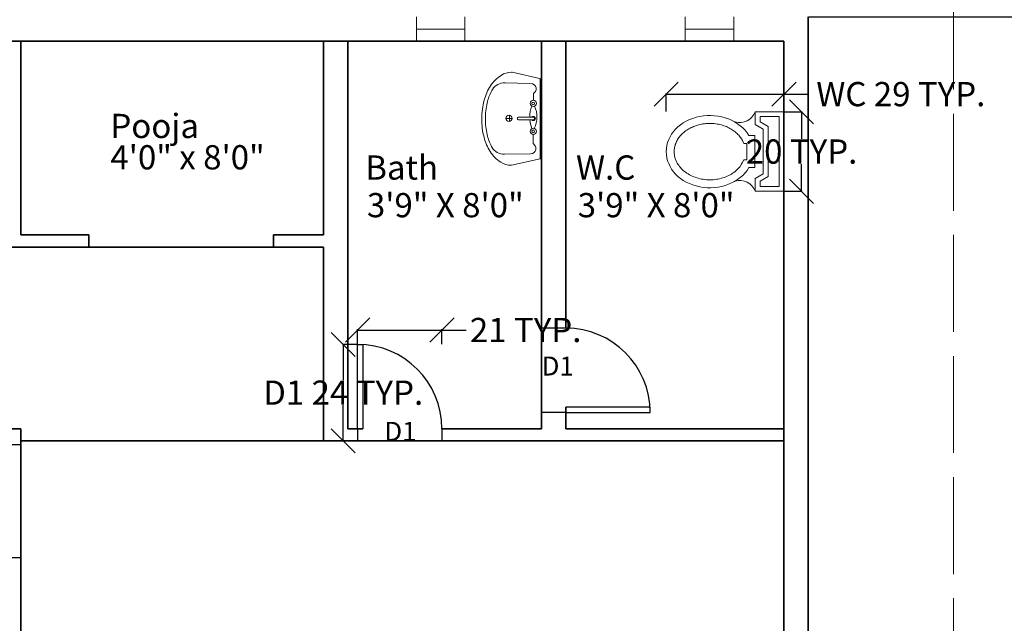
# Model space of a CAD drawing. Units: inches. Extents: x -1198 to -69, y -512 to 437.
# Tile 48 of 50: x -566 to -322, y 113 to 263. Entities that reach past the tile are written whole.
import ezdxf

# ---------------------------------------------------------------- set-up
doc = ezdxf.new("R2010")
doc.units = ezdxf.units.IN
doc.header["$MEASUREMENT"] = 0
doc.linetypes.add('ACAD_ISO02W100', pattern=[15, 12, -3])
for name, color, linetype, lineweight in [('A-ANNO-DIMS', 2, 'Continuous', 18), ('A-ANNO-SYMB', 7, 'Continuous', 18), ('A-AREA-IDEN', 7, 'Continuous', 18), ('A-FLOR-FIXT', 60, 'Continuous', 18), ('A-WALL', 7, 'Continuous', 35), ('C-PROP', 141, 'ACAD_ISO02W100', 18), ('Doors', 140, 'Continuous', 25), ('windows', 160, 'Continuous', 18)]:
    doc.layers.add(name, color=color, linetype=linetype, lineweight=lineweight)
doc.styles.get("Standard").update_dxf_attribs({"font": 'arial.ttf'})
doc.dimstyles.get("Standard").update_dxf_attribs({"dimtxt": 6, "dimasz": 6, "dimexe": 0.18, "dimexo": 0.0625, "dimgap": 0.09, "dimtad": 0, "dimtih": 1, "dimtoh": 1, "dimdec": 0, "dimzin": 0, "dimdsep": 46, "dimlunit": 4, "dimtxsty": 'Standard', "dimblk": 'OBLIQUE', "dimcen": 0.09, "dimadec": 0, "dimazin": 0, "dimtfac": 1, "dimtdec": 0, "dimtofl": 0, "dimtmove": 0, "dimatfit": 3, "dimfxl": 1, "dimtolj": 1, "dimtzin": 0, "dimarcsym": 0})

# ---------------------------------------------------------------- blocks, each defined once
blk = doc.blocks.new('*U4')
for p, q in [((0, 0), (0, -6)), ((28, 0), (28, -6))]:
    blk.add_line(p, q)
blk.add_lwpolyline([(0, 0), (0, 28), (1.75, 28), (1.75, 0)], close=True)
blk.add_arc((0, 0), 28, 0, 90)
blk = doc.blocks.new('A$C7C8779AE')
for p, q in [((0, 0.7405), (0, 0.5605)), ((0.5, 0.7405), (0, 0.7405)), ((0.47, 0.7105), (0.03, 0.7105)), ((0.03, 0.7105), (0.03, 0.5905)), ((0.47, 0.5905), (0.47, 0.7105)), ((0.5, 0.5605), (0.5, 0.7405)), ((0.093, 0.6405), (0.063, 0.5905)), ((0.093, 0.6405), (0.407, 0.6405)), ((0.437, 0.5905), (0.407, 0.6405)), ((0, 0.5605), (0.08, 0.5605)), ((0.03, 0.5905), (0.063, 0.5905)), ((0.11, 0.6105), (0.08, 0.5605)), ((0.11, 0.6105), (0.39, 0.6105)), ((0.42, 0.5605), (0.39, 0.6105)), ((0.42, 0.5605), (0.5, 0.5605)), ((0.437, 0.5905), (0.47, 0.5905)), ((0.1497, 0.557), (0.1497, 0.5203)), ((0.1497, 0.557), (0.3514, 0.557)), ((0.1997, 0.507), (0.1997, 0.4879)), ((0.1997, 0.507), (0.3014, 0.507)), ((0.3014, 0.507), (0.3014, 0.4879)), ((0.3514, 0.557), (0.3514, 0.5203))]:
    blk.add_line(p, q)
for centre, start, end in [((-0.0386, 0.4613), 344.64203, 68.73386), ((0.5386, 0.4613), 111.26614, 195.35797)]:
    blk.add_arc(centre, 0.1064, start, end)
blk.add_ellipse((0.2506, 0.2744), major_axis=(0, 0.2744), ratio=0.828948, start_param=0.459479, end_param=5.823706)
blk.add_open_spline([(0.1997, 0.4879), (0.1697, 0.474), (0.1642, 0.4702), (0.1512, 0.4602), (0.1438, 0.4535), (0.1298, 0.4388), (0.1233, 0.4306), (0.1111, 0.4131), (0.1055, 0.4037), (0.0956, 0.3838), (0.0912, 0.3733), (0.0838, 0.3516), (0.0808, 0.3403), (0.0762, 0.3172), (0.0746, 0.3055), (0.073, 0.2817), (0.0729, 0.2698), (0.0743, 0.246), (0.0758, 0.2342), (0.0801, 0.2111), (0.0831, 0.1998), (0.0903, 0.1779), (0.0945, 0.1673), (0.1043, 0.1473), (0.1098, 0.1378), (0.1218, 0.12), (0.1283, 0.1118), (0.1421, 0.0968), (0.1494, 0.09), (0.1646, 0.078), (0.1725, 0.0728), (0.1887, 0.064), (0.1969, 0.0603), (0.2137, 0.0547), (0.2222, 0.0527), (0.2392, 0.0502), (0.2478, 0.0498), (0.2664, 0.0505), (0.2764, 0.052), (0.2963, 0.0573), (0.3061, 0.061), (0.3253, 0.0707), (0.3346, 0.0766), (0.3525, 0.0906), (0.3611, 0.0987), (0.3771, 0.1169), (0.3845, 0.127), (0.3978, 0.1488), (0.4037, 0.1605), (0.4137, 0.1853), (0.4178, 0.1983), (0.424, 0.2251), (0.4261, 0.2389), (0.4282, 0.2668), (0.4283, 0.2809), (0.4262, 0.3088), (0.4241, 0.3226), (0.418, 0.3495), (0.414, 0.3625), (0.404, 0.3873), (0.3982, 0.3991), (0.385, 0.421), (0.3776, 0.4311), (0.3617, 0.4494), (0.3531, 0.4575), (0.3382, 0.4693), (0.3321, 0.4736), (0.3014, 0.4879)], degree=3, knots=[0.459479, 0.459479, 0.459479, 0.459479, 0.567422, 0.567422, 0.720865, 0.720865, 0.874307, 0.874307, 1.02775, 1.02775, 1.181192, 1.181192, 1.334635, 1.334635, 1.488077, 1.488077, 1.64152, 1.64152, 1.794963, 1.794963, 1.948405, 1.948405, 2.101848, 2.101848, 2.25529, 2.25529, 2.408733, 2.408733, 2.562175, 2.562175, 2.715618, 2.715618, 2.86906, 2.86906, 3.022503, 3.022503, 3.175946, 3.175946, 3.356457, 3.356457, 3.536968, 3.536968, 3.717479, 3.717479, 3.89799, 3.89799, 4.078501, 4.078501, 4.259012, 4.259012, 4.439523, 4.439523, 4.620035, 4.620035, 4.800546, 4.800546, 4.981057, 4.981057, 5.161568, 5.161568, 5.342079, 5.342079, 5.52259, 5.52259, 5.703101, 5.703101, 5.823706, 5.823706, 5.823706, 5.823706])
blk = doc.blocks.new('A')
at = {"xscale": 1000, "yscale": 1000, "zscale": 1000}
blk.add_blockref('A$C7C8779AE', (-250.6, 0), dxfattribs=at)
blk = doc.blocks.new('A$C6AA41FE3')
at = {"linetype": 'ByBlock'}
for p, q in [((0.1919, 0.5849), (0.3733, 0.5439)), ((0.3026, 0.514), (0.1469, 0.5187)), ((0.32, 0.5127), (0.3026, 0.514)), ((0.3305, 0.5069), (0.32, 0.5127)), ((0.3383, 0.4979), (0.3305, 0.5069)), ((0.3425, 0.4869), (0.3383, 0.4979)), ((0.3687, 0.04), (0.3687, 0.5439)), ((0.3687, 0.5439), (0.3772, 0.5439)), ((0.3772, 0.0411), (0.3772, 0.5439)), ((0.3251, 0.409), (0.3253, 0.4524)), ((0.3253, 0.4524), (0.3305, 0.4553)), ((0.3305, 0.4553), (0.3383, 0.4642)), ((0.3383, 0.4642), (0.3425, 0.4752)), ((0.3425, 0.4752), (0.3425, 0.4869)), ((0.1747, 0.3146), (0.1747, 0.2774)), ((0.1525, 0.2951), (0.1884, 0.2951)), ((0.2326, 0.3025), (0.3243, 0.3025)), ((0.2326, 0.3021), (0.2326, 0.3025)), ((0.2326, 0.2863), (0.2326, 0.2867)), ((0.3243, 0.2863), (0.2326, 0.2863)), ((0.3243, 0.3025), (0.3243, 0.3024)), ((0.3243, 0.2864), (0.3243, 0.2863)), ((0.3243, 0.1379), (0.3245, 0.1941)), ((0.3374, 0.1229), (0.3243, 0.1379)), ((0.144, 0.0693), (0.3071, 0.0724)), ((0.3071, 0.0724), (0.3191, 0.0744)), ((0.3191, 0.0744), (0.3296, 0.0802)), ((0.3296, 0.0802), (0.3374, 0.0892)), ((0.3415, 0.1119), (0.3374, 0.1229)), ((0.3374, 0.0892), (0.3415, 0.1002)), ((0.3415, 0.1002), (0.3415, 0.1119)), ((0.188, 0), (0.3687, 0.04)), ((0.3772, 0.0411), (0.3687, 0.0411))]:
    blk.add_line(p, q, dxfattribs=at)
for centre, radius in [((0.3245, 0.3895), 0.0195), ((0.3245, 0.3895), 0.00849), ((0.172, 0.2951), 0.0195), ((0.3245, 0.2136), 0.0195), ((0.3245, 0.2136), 0.00849)]:
    blk.add_circle(centre, radius, dxfattribs=at)
for centre, radius, start, end in [((0.241, 0.3799), 0.2208, 122.64614, 147.09358), ((0.1864, 0.4671), 0.118, 89.17847, 123.14131), ((0.1877, 0.4667), 0.1183, 87.92664, 89.81125), ((0.3304, 0.324), 0.3262, 147.38302, 164.68206), ((0.1441, 0.4288), 0.09, 88.25949, 147.75883), ((0.3272, 0.3256), 0.3003, 152.13058, 167.30015), ((0.2193, 0.3814), 0.1789, 147.75883, 151.77231), ((0.4743, 0.289), 0.4743, 165.19563, 179.4863), ((0.5, 0.2906), 0.4766, 167.76557, 179.77021), ((0.1798, 0.3042), 0.1678, 334.48749, 24.17939), ((0.4839, 0.3016), 0.1818, 157.46452, 179.70612), ((0.4743, 0.2935), 0.4743, 180.03161, 194.32228), ((0.5, 0.2944), 0.4766, 180.22979, 192.23443), ((0.2312, 0.2944), 0.0078, 80.15507, 279.84493), ((0.4839, 0.3016), 0.1818, 184.80871, 202.53548), ((0.3243, 0.2944), 0.013, 218.4979, 141.5021), ((0.3243, 0.2944), 0.0134, 270, 90), ((0.3243, 0.2944), 0.00798, 270, 90), ((0.3272, 0.2594), 0.3003, 192.69985, 207.86942), ((0.33, 0.2597), 0.3262, 194.84096, 212.14001), ((0.2402, 0.2046), 0.2208, 212.44128, 236.88872), ((0.2193, 0.2037), 0.1789, 208.22812, 209.97994), ((0.1423, 0.1592), 0.09, 209.97994, 271.05374), ((0.1848, 0.1179), 0.1179, 236.40841, 270.37125), ((0.1861, 0.1183), 0.1183, 269.7541, 270.94709)]:
    blk.add_arc(centre, radius, start, end, dxfattribs=at)
blk = doc.blocks.new('A1')
at = {"xscale": 1000, "yscale": 1000, "zscale": 1000, "rotation": 90}
blk.add_blockref('A$C6AA41FE3', (292.5, -377.2), dxfattribs=at)
blk = doc.blocks.new('VENT-12')
at = {"ltscale": 10}
for p, q in [((0, 6), (0, 0)), ((12, 6), (12, 0)), ((0, 3), (12, 3))]:
    blk.add_line(p, q, dxfattribs=at)
blk = doc.blocks.new('DOOR-D1-JAMB3')
for p, q in [((0, 0), (0, -3)), ((20.87, 0), (20.87, -3))]:
    blk.add_line(p, q)
blk.add_lwpolyline([(0, 0), (0, 20.87), (1.3, 20.87), (1.3, 0)], close=True)
blk.add_arc((0, 0), 20.87, 0, 90)
blk = doc.blocks.new('DOOR-D1-JAMB6')
for p, q in [((0, 20.87), (-6, 20.87)), ((0, 0), (-6, 0))]:
    blk.add_line(p, q)
blk.add_lwpolyline([(0, 0), (20.87, 0), (20.87, 1.3), (0, 1.3)], close=True)
blk.add_arc((0, 0), 20.87, 0, 90)
blk = doc.blocks.new('_Oblique')
at = {"color": 0, "linetype": 'ByBlock', "lineweight": -2}
blk.add_line((-0.5, -0.5), (0.5, 0.5), dxfattribs=at)
blk = doc.blocks.new('*D32')
at = {"layer": 'A-ANNO-DIMS', "color": 0, "lineweight": -2, "ltscale": 10, "transparency": 16777216}
for p, q in [((-482.38, 182.1), (-486.08, 182.1)), ((-485.9, 182.1), (-485.9, 173.27)), ((-485.9, 158.23), (-485.9, 167.06)), ((-482.38, 158.23), (-486.08, 158.23))]:
    blk.add_line(p, q, dxfattribs=at)
at = {"layer": 'DEFPOINTS', "color": 0, "ltscale": 10, "transparency": 16777216}
for p in [(-485.9, 182.1), (-482.32, 182.1), (-482.32, 158.23)]:
    blk.add_point(p, dxfattribs=at)
at = {"layer": 'A-ANNO-DIMS', "color": 0, "lineweight": -2, "ltscale": 10, "transparency": 16777216, "xscale": 6, "yscale": 6, "zscale": 6}
for p, rotation in [((-485.9, 182.1), 90), ((-485.9, 158.23), 270)]:
    blk.add_blockref('_Oblique', p, dxfattribs=dict(at, rotation=rotation))
at = {"layer": 'A-ANNO-DIMS', "color": 0, "ltscale": 10, "transparency": 16777216, "insert": (-485.9, 170.16), "char_height": 6, "attachment_point": 5}
blk.add_mtext('\\A1;D1 24 TYP.', dxfattribs=at)
blk = doc.blocks.new('*D33')
at = {"layer": 'A-ANNO-DIMS', "color": 0, "lineweight": -2, "ltscale": 10, "transparency": 16777216}
for p, q in [((-482.32, 182.16), (-482.32, 185.86)), ((-482.32, 185.68), (-461.45, 185.68)), ((-461.45, 182.16), (-461.45, 185.86)), ((-461.45, 185.68), (-455.45, 185.68))]:
    blk.add_line(p, q, dxfattribs=at)
at = {"layer": 'DEFPOINTS', "color": 0, "ltscale": 10, "transparency": 16777216}
for p in [(-461.45, 185.68), (-482.32, 182.1), (-461.45, 182.1)]:
    blk.add_point(p, dxfattribs=at)
at = {"layer": 'A-ANNO-DIMS', "color": 0, "lineweight": -2, "ltscale": 10, "transparency": 16777216, "xscale": 6, "yscale": 6, "zscale": 6, "rotation": 180}
blk.add_blockref('_Oblique', (-482.32, 185.68), dxfattribs=at)
at = {"layer": 'A-ANNO-DIMS', "color": 0, "lineweight": -2, "ltscale": 10, "transparency": 16777216, "xscale": 6, "yscale": 6, "zscale": 6}
blk.add_blockref('_Oblique', (-461.45, 185.68), dxfattribs=at)
at = {"layer": 'A-ANNO-DIMS', "color": 0, "ltscale": 10, "transparency": 16777216, "insert": (-440.71, 185.68), "char_height": 6, "attachment_point": 5}
blk.add_mtext('\\A1;21 TYP.', dxfattribs=at)
blk = doc.blocks.new('*D42')
at = {"layer": 'A-ANNO-DIMS', "color": 0, "lineweight": -2, "ltscale": 10, "transparency": 16777216}
for p, q in [((-405.9, 239.8), (-405.9, 244.29)), ((-405.9, 244.11), (-376.75, 244.11)), ((-376.75, 239.8), (-376.75, 244.29)), ((-376.75, 244.11), (-370.75, 244.11))]:
    blk.add_line(p, q, dxfattribs=at)
at = {"layer": 'DEFPOINTS', "color": 0, "ltscale": 10, "transparency": 16777216}
for p in [(-376.75, 244.11), (-405.9, 239.73), (-376.75, 239.73)]:
    blk.add_point(p, dxfattribs=at)
at = {"layer": 'A-ANNO-DIMS', "color": 0, "lineweight": -2, "ltscale": 10, "transparency": 16777216, "xscale": 6, "yscale": 6, "zscale": 6, "rotation": 180}
blk.add_blockref('_Oblique', (-405.9, 244.11), dxfattribs=at)
at = {"layer": 'A-ANNO-DIMS', "color": 0, "lineweight": -2, "ltscale": 10, "transparency": 16777216, "xscale": 6, "yscale": 6, "zscale": 6}
blk.add_blockref('_Oblique', (-376.75, 244.11), dxfattribs=at)
at = {"layer": 'A-ANNO-DIMS', "color": 0, "ltscale": 10, "transparency": 16777216, "insert": (-347.79, 244.11), "char_height": 6, "attachment_point": 5}
blk.add_mtext('\\A1;WC 29 TYP.', dxfattribs=at)
blk = doc.blocks.new('*D43')
at = {"layer": 'A-ANNO-DIMS', "color": 0, "lineweight": -2, "ltscale": 10, "transparency": 16777216}
for p, q in [((-376.69, 239.73), (-372.2, 239.73)), ((-372.38, 239.73), (-372.38, 233.04)), ((-372.38, 220.05), (-372.38, 226.74)), ((-376.69, 220.05), (-372.2, 220.05))]:
    blk.add_line(p, q, dxfattribs=at)
at = {"layer": 'DEFPOINTS', "color": 0, "ltscale": 10, "transparency": 16777216}
for p in [(-376.75, 239.73), (-376.75, 220.05), (-372.38, 220.05)]:
    blk.add_point(p, dxfattribs=at)
at = {"layer": 'A-ANNO-DIMS', "color": 0, "lineweight": -2, "ltscale": 10, "transparency": 16777216, "xscale": 6, "yscale": 6, "zscale": 6}
for p, rotation in [((-372.38, 239.73), 90), ((-372.38, 220.05), 270)]:
    blk.add_blockref('_Oblique', p, dxfattribs=dict(at, rotation=rotation))
at = {"layer": 'A-ANNO-DIMS', "color": 0, "ltscale": 10, "transparency": 16777216, "insert": (-372.38, 229.89), "char_height": 6, "attachment_point": 5}
blk.add_mtext('\\A1;20 TYP.', dxfattribs=at)
blk = doc.blocks.new('*D63')
at = {"layer": 'A-ANNO-DIMS', "color": 0, "lineweight": -2, "ltscale": 10, "transparency": 16777216}
for p, q in [((-370.69, 263.23), (-79.37, 263.23)), ((-79.55, 263.23), (-79.55, 20.38)), ((-79.55, -228.77), (-79.55, 14.07)), ((-370.69, -228.77), (-79.37, -228.77))]:
    blk.add_line(p, q, dxfattribs=at)
at = {"layer": 'DEFPOINTS', "color": 0, "ltscale": 10, "transparency": 16777216}
for p in [(-370.75, 263.23), (-79.55, 263.23), (-370.75, -228.77)]:
    blk.add_point(p, dxfattribs=at)
at = {"layer": 'A-ANNO-DIMS', "color": 0, "lineweight": -2, "ltscale": 10, "transparency": 16777216, "xscale": 6, "yscale": 6, "zscale": 6}
for p, rotation in [((-79.55, 263.23), 90), ((-79.55, -228.77), 270)]:
    blk.add_blockref('_Oblique', p, dxfattribs=dict(at, rotation=rotation))
at = {"layer": 'A-ANNO-DIMS', "color": 0, "ltscale": 10, "transparency": 16777216, "insert": (-79.55, 17.23), "char_height": 6, "attachment_point": 5}
blk.add_mtext('\\A1;492', dxfattribs=at)

msp = doc.modelspace()

# ---------------------------------------------------------------- linework, layer by layer
at = {"layer": 'A-WALL', "ltscale": 10}
for p, q in [((-370.7509, -228.7723), (-370.7509, 263.2277)), ((-376.7509, 257.2277), (-691.7509, 257.2277)), ((-490.7509, 257.2277), (-565.7509, 257.2277)), ((-565.7509, 257.2277), (-565.7509, 209.2277)), ((-490.7509, 257.2277), (-490.7509, 209.2277)), ((-436.7509, 257.2277), (-484.7509, 257.2277)), ((-484.7509, 257.2277), (-484.7509, 161.2277)), ((-436.7509, 257.2277), (-436.7509, 161.2277)), ((-376.7509, 257.2277), (-430.7509, 257.2277)), ((-430.7509, 257.2277), (-430.7509, 186.149)), ((-376.7509, -222.7723), (-376.7509, 257.2277)), ((-548.9135, 209.2277), (-565.7509, 209.2277)), ((-548.9135, 209.2277), (-548.9135, 206.2277)), ((-490.7509, 209.2277), (-503.1219, 209.2277)), ((-503.1219, 209.2277), (-503.1219, 206.2277)), ((-490.7509, 206.2277), (-571.7509, 206.2277)), ((-490.7509, 206.2277), (-490.7509, 161.2277)), ((-430.7509, 166.5837), (-430.7509, 161.2277)), ((-565.7509, 161.2277), (-691.7509, 161.2277)), ((-565.7509, 161.2277), (-565.7509, 35.2277)), ((-490.7509, 161.2277), (-490.7509, 158.2277)), ((-481.0154, 161.2277), (-484.7509, 161.2277)), ((-436.7509, 161.2277), (-461.4501, 161.2277)), ((-376.7509, 161.2277), (-430.7509, 161.2277)), ((-376.7509, 158.2277), (-565.7509, 158.2277))]:
    msp.add_line(p, q, dxfattribs=at)
at = {"layer": 'C-PROP', "ltscale": 2}
msp.add_lwpolyline([(-1054.7509, 299.2277), (-334.7509, 299.2277), (-334.7509, -264.7723), (-1054.7509, -264.7723)], close=True, dxfattribs=at)

# ---------------------------------------------------------------- block references
at = {"layer": 'A-FLOR-FIXT', "ltscale": 10, "xscale": 0.0393700787401575, "yscale": 0.0393700787401575, "zscale": 0.0393700787401575, "rotation": 270}
for name, p in [('A1', (-436.7509, 237.9979)), ('A', (-405.9029, 229.8684))]:
    msp.add_blockref(name, p, dxfattribs=at)
at = {"layer": 'Doors'}
for name, p in [('DOOR-D1-JAMB6', (-430.7509, 165.2794)), ('DOOR-D1-JAMB3', (-482.3198, 161.2277)), ('DOOR-D1-JAMB3', (-482.3198, 161.2277))]:
    msp.add_blockref(name, p, dxfattribs=at)
at = {"layer": 'Doors', "xscale": -1, "rotation": 90}
msp.add_blockref('*U4', (-571.7509, 157.3222), dxfattribs=at)
at = {"layer": 'windows', "rotation": 180}
for p in [(-455.7361, 263.2273), (-389.1785, 263.2273)]:
    msp.add_blockref('VENT-12', p, dxfattribs=at)

# ---------------------------------------------------------------- texts
at = {"layer": 'A-ANNO-SYMB', "ltscale": 10}
for p in [(-436.7509, 174.4049), (-475.7071, 158.2277)]:
    msp.add_text('D1', height=4.69957, dxfattribs=at).set_placement(p)
at = {"layer": 'A-AREA-IDEN', "ltscale": 10, "char_height": 6, "attachment_point": 1}
for s, insert in [('Pooja', (-543.5573, 239.2277)), ('4\'0" x 8\'0"', (-543.5573, 231.4637)), ('Bath', (-480.4421, 228.9301)), ('W.C', (-428.2349, 228.9301)), ('3\'9" X 8\'0"', (-480.0227, 219.603)), ('3\'9" X 8\'0"', (-427.8154, 219.603))]:
    msp.add_mtext_dynamic_manual_height_columns(s, width=57.976527, gutter_width=30, heights=[0], dxfattribs=dict(at, insert=insert))

# ---------------------------------------------------------------- dimensions: what is measured, and where the dimension line sits
at = {"layer": 'A-ANNO-DIMS', "ltscale": 10}
dim = msp.add_linear_dim(base=(-79.5507, 263.2277), p1=(-370.7509, -228.7723), p2=(-370.7509, 263.2277), angle=90, dimstyle='Standard', override={"dimdec": 0, "dimlfac": 1, "dimrnd": 0, "dimzin": 0, "dimdsep": 46, "dimlunit": 2}, dxfattribs=at)
dim.commit()
dim.dimension.update_dxf_attribs({"geometry": '*D63', "text_midpoint": (-79.5507, 17.2277)})
for base, p1, p2, text, picture, middle in [((-376.7509, 244.1058), (-405.9029, 239.733), (-376.7509, 239.733), 'WC <> TYP.', '*D42', (-347.7884, 244.1058)), ((-461.4501, 185.6778), (-482.3198, 182.0973), (-461.4501, 182.0973), '<> TYP.', '*D33', (-440.7059, 185.6778))]:
    dim = msp.add_linear_dim(base=base, p1=p1, p2=p2, text=text, dimstyle='Standard', override={"dimdec": 0, "dimlfac": 1, "dimrnd": 0, "dimzin": 0, "dimdsep": 46, "dimlunit": 2}, dxfattribs=at)
    dim.commit()
    dim.dimension.update_dxf_attribs({"geometry": picture, "text_midpoint": middle})
for base, p1, p2, angle, text, picture, middle in [((-372.3781, 220.048), (-376.7509, 239.733), (-376.7509, 220.048), 270, '<> TYP.', '*D43', (-372.3781, 229.8905)), ((-485.9002, 182.0973), (-482.3198, 158.2277), (-482.3198, 182.0973), 90, 'D1 <> TYP.', '*D32', (-485.9002, 170.1625))]:
    dim = msp.add_linear_dim(base=base, p1=p1, p2=p2, angle=angle, text=text, dimstyle='Standard', override={"dimdec": 0, "dimlfac": 1, "dimrnd": 0, "dimzin": 0, "dimdsep": 46, "dimlunit": 2}, dxfattribs=at)
    dim.commit()
    dim.dimension.update_dxf_attribs({"geometry": picture, "text_midpoint": middle})

doc.saveas('drawing.dxf')
